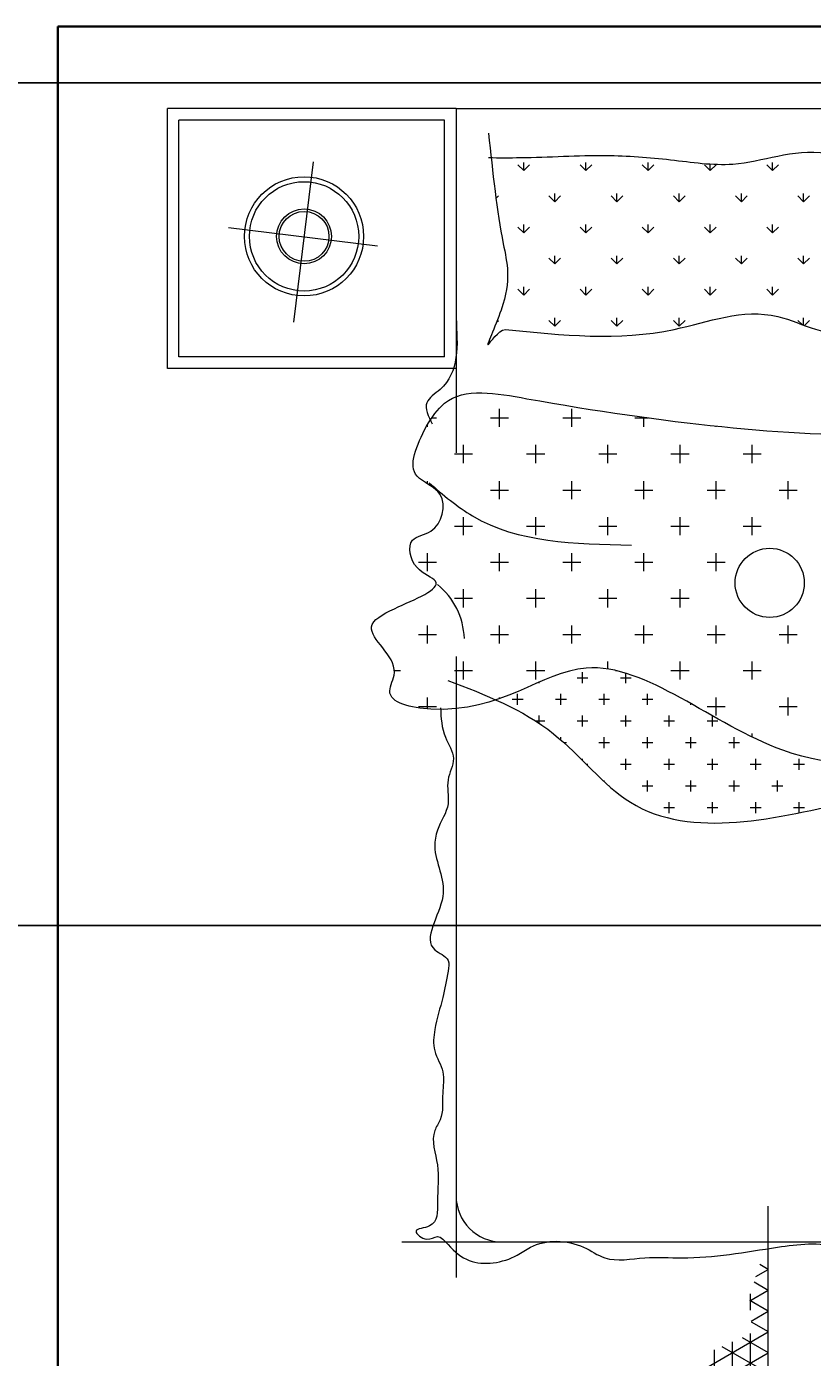
# Model space of a CAD drawing. Units: inches. Extents: x 3731 to 4318, y 1310 to 2388.
# Tile 26 of 57: x 3838 to 3894, y 1844 to 1938. Entities that reach past the tile are written whole.
import ezdxf

# ---------------------------------------------------------------- set-up
doc = ezdxf.new("R2010")
doc.units = ezdxf.units.IN
for name, color, linetype, lineweight in [('A-ANNO-DIMS', 2, 'Continuous', 18), ('A-FURN', 8, 'Continuous', 13), ('A-WALL', 7, 'Continuous', 35)]:
    doc.layers.add(name, color=color, linetype=linetype, lineweight=lineweight)
doc.styles.get("Standard").update_dxf_attribs({"font": 'arial.ttf'})
doc.dimstyles.get("Standard").update_dxf_attribs({"dimtxt": 0.18, "dimasz": 0.18, "dimexe": 0.18, "dimexo": 0.0625, "dimgap": 0.09, "dimtad": 0, "dimtih": 1, "dimtoh": 1, "dimdec": 4, "dimzin": 0, "dimdsep": 46, "dimtxsty": 'Standard', "dimcen": 0.09, "dimadec": 0, "dimazin": 0, "dimtfac": 1, "dimtdec": 4, "dimtofl": 0, "dimtmove": 0, "dimatfit": 3, "dimfxl": 1, "dimtolj": 1, "dimtzin": 0, "dimarcsym": 0})

# ---------------------------------------------------------------- blocks, each defined once
blk = doc.blocks.new('A$C200C7901')
for p, q in [((0, 1.8834), (0, 2.3334)), ((0.5, 2.3334), (0, 2.3334)), ((0.5, 2.3334), (0.5, 1.7369)), ((0.5, 2.3334), (0.5, 1.7369)), ((0.5, 2.3334), (2, 2.3334)), ((0.9943, 2.1721), (0.9842, 2.1822)), ((0.9943, 2.1721), (0.9842, 2.1822)), ((0.9943, 2.0643), (0.9842, 2.0744)), ((0.9943, 2.0643), (0.9842, 2.0744)), ((0.5701, 1.9635), (0.5733, 1.9666)), ((0.5701, 1.9635), (0.5733, 1.9666)), ((0.5, 1.8834), (0, 1.8834)), ((0.4504, 1.782), (0.4504, 1.7863)), ((0.4504, 1.782), (0.4504, 1.7863)), ((0.458, 1.7977), (0.466, 1.7977)), ((0.458, 1.7977), (0.466, 1.7977)), ((0.4504, 1.6834), (0.4504, 1.6883)), ((0.4504, 1.6834), (0.4504, 1.6883)), ((0.4656, 1.6727), (0.466, 1.6727)), ((0.4656, 1.6727), (0.466, 1.6727)), ((0.5597, 1.6727), (0.591, 1.6727)), ((0.5597, 1.6727), (0.591, 1.6727)), ((1.0129, 1.5945), (1.0129, 1.6258)), ((1.0129, 1.5945), (1.0129, 1.6258)), ((0.4347, 1.5477), (0.466, 1.5477)), ((0.4504, 1.532), (0.4504, 1.5633)), ((0.6847, 1.5477), (0.716, 1.5477)), ((1.0754, 1.5625), (1.0754, 1.5633)), ((1.0754, 1.5625), (1.0754, 1.5633)), ((0.4347, 1.4227), (0.466, 1.4227)), ((0.5, 1.3845), (0.5, 0.3086)), ((0.3931, 1.3602), (0.4035, 1.3602)), ((0.3931, 1.3602), (0.4035, 1.3602)), ((0.4972, 1.3602), (0.5285, 1.3602)), ((0.4972, 1.3602), (0.5285, 1.3602)), ((0.4347, 1.2977), (0.466, 1.2977)), ((0.4347, 1.2977), (0.466, 1.2977)), ((0.4504, 1.2936), (0.4504, 1.3133)), ((0.4504, 1.2936), (0.4504, 1.3133)), ((1.0407, 0.0275), (1.0407, 0.4323)), ((0.4061, 0.3703), (2.0386, 0.3703))]:
    blk.add_line(p, q)
at = {"linetype": 'ByBlock'}
for p, q in [((0.02, 1.9034), (0.02, 2.3134)), ((0.48, 2.3134), (0.02, 2.3134)), ((0.48, 1.9034), (0.48, 2.3134)), ((0.2524, 2.2412), (0.2186, 1.9635)), ((0.6171, 2.2259), (0.607, 2.236)), ((0.6171, 2.2259), (0.607, 2.236)), ((0.6171, 2.2259), (0.6171, 2.2402)), ((0.6171, 2.2259), (0.6171, 2.2402)), ((0.6171, 2.2259), (0.6272, 2.236)), ((0.6171, 2.2259), (0.6272, 2.236)), ((0.7249, 2.2259), (0.7148, 2.236)), ((0.7249, 2.2259), (0.7148, 2.236)), ((0.7249, 2.2259), (0.7249, 2.2402)), ((0.7249, 2.2259), (0.7249, 2.2402)), ((0.7249, 2.2259), (0.735, 2.236)), ((0.7249, 2.2259), (0.735, 2.236)), ((0.8326, 2.2259), (0.8225, 2.236)), ((0.8326, 2.2259), (0.8225, 2.236)), ((0.8326, 2.2259), (0.8326, 2.2402)), ((0.8326, 2.2259), (0.8326, 2.2402)), ((0.8326, 2.2259), (0.8427, 2.236)), ((0.8326, 2.2259), (0.8427, 2.236)), ((0.9404, 2.2259), (0.9303, 2.236)), ((0.9404, 2.2259), (0.9303, 2.236)), ((0.9404, 2.2259), (0.9404, 2.2369)), ((0.9404, 2.2259), (0.9404, 2.2369)), ((0.9404, 2.2259), (0.9505, 2.236)), ((0.9404, 2.2259), (0.9505, 2.236)), ((1.0482, 2.2259), (1.0381, 2.236)), ((1.0482, 2.2259), (1.0381, 2.236)), ((1.0482, 2.2259), (1.0482, 2.2402)), ((1.0482, 2.2259), (1.0482, 2.2402)), ((1.0482, 2.2259), (1.0583, 2.236)), ((1.0482, 2.2259), (1.0583, 2.236)), ((0.5692, 2.178), (0.5733, 2.1822)), ((0.5692, 2.178), (0.5733, 2.1822)), ((0.671, 2.1721), (0.6609, 2.1822)), ((0.671, 2.1721), (0.6609, 2.1822)), ((0.671, 2.172), (0.671, 2.1863)), ((0.671, 2.172), (0.671, 2.1863)), ((0.671, 2.1721), (0.6811, 2.1822)), ((0.671, 2.1721), (0.6811, 2.1822)), ((0.7787, 2.1721), (0.7686, 2.1822)), ((0.7787, 2.1721), (0.7686, 2.1822)), ((0.7787, 2.172), (0.7787, 2.1863)), ((0.7787, 2.172), (0.7787, 2.1863)), ((0.7787, 2.1721), (0.7889, 2.1822)), ((0.7787, 2.1721), (0.7889, 2.1822)), ((0.8865, 2.1721), (0.8764, 2.1822)), ((0.8865, 2.1721), (0.8764, 2.1822)), ((0.8865, 2.172), (0.8865, 2.1863)), ((0.8865, 2.172), (0.8865, 2.1863)), ((0.8865, 2.1721), (0.8966, 2.1822)), ((0.8865, 2.1721), (0.8966, 2.1822)), ((0.9943, 2.172), (0.9943, 2.1863)), ((0.9943, 2.172), (0.9943, 2.1863)), ((0.9943, 2.1721), (1.0044, 2.1822)), ((0.9943, 2.1721), (1.0044, 2.1822)), ((1.102, 2.1721), (1.0919, 2.1822)), ((1.102, 2.1721), (1.0919, 2.1822)), ((1.102, 2.172), (1.102, 2.1863)), ((1.102, 2.172), (1.102, 2.1863)), ((1.102, 2.1721), (1.1121, 2.1822)), ((1.102, 2.1721), (1.1121, 2.1822)), ((0.3641, 2.0951), (0.1061, 2.1268)), ((0.6171, 2.1182), (0.607, 2.1283)), ((0.6171, 2.1182), (0.607, 2.1283)), ((0.6171, 2.1182), (0.6171, 2.1325)), ((0.6171, 2.1182), (0.6171, 2.1325)), ((0.6171, 2.1182), (0.6272, 2.1283)), ((0.6171, 2.1182), (0.6272, 2.1283)), ((0.7249, 2.1182), (0.7148, 2.1283)), ((0.7249, 2.1182), (0.7148, 2.1283)), ((0.7249, 2.1182), (0.7249, 2.1325)), ((0.7249, 2.1182), (0.7249, 2.1325)), ((0.7249, 2.1182), (0.735, 2.1283)), ((0.7249, 2.1182), (0.735, 2.1283)), ((0.8326, 2.1182), (0.8225, 2.1283)), ((0.8326, 2.1182), (0.8225, 2.1283)), ((0.8326, 2.1182), (0.8326, 2.1325)), ((0.8326, 2.1182), (0.8326, 2.1325)), ((0.8326, 2.1182), (0.8427, 2.1283)), ((0.8326, 2.1182), (0.8427, 2.1283)), ((0.9404, 2.1182), (0.9303, 2.1283)), ((0.9404, 2.1182), (0.9303, 2.1283)), ((0.9404, 2.1182), (0.9404, 2.1325)), ((0.9404, 2.1182), (0.9404, 2.1325)), ((0.9404, 2.1182), (0.9505, 2.1283)), ((0.9404, 2.1182), (0.9505, 2.1283)), ((1.0482, 2.1182), (1.0381, 2.1283)), ((1.0482, 2.1182), (1.0381, 2.1283)), ((1.0482, 2.1182), (1.0482, 2.1325)), ((1.0482, 2.1182), (1.0482, 2.1325)), ((1.0482, 2.1182), (1.0583, 2.1283)), ((1.0482, 2.1182), (1.0583, 2.1283)), ((0.671, 2.0643), (0.671, 2.0786)), ((0.671, 2.0643), (0.671, 2.0786)), ((0.7787, 2.0643), (0.7787, 2.0786)), ((0.7787, 2.0643), (0.7787, 2.0786)), ((0.8865, 2.0643), (0.8865, 2.0786)), ((0.8865, 2.0643), (0.8865, 2.0786)), ((0.9943, 2.0643), (0.9943, 2.0786)), ((0.9943, 2.0643), (0.9943, 2.0786)), ((1.102, 2.0643), (1.102, 2.0786)), ((1.102, 2.0643), (1.102, 2.0786)), ((0.671, 2.0643), (0.6609, 2.0744)), ((0.671, 2.0643), (0.6609, 2.0744)), ((0.671, 2.0643), (0.6811, 2.0744)), ((0.671, 2.0643), (0.6811, 2.0744)), ((0.7787, 2.0643), (0.7686, 2.0744)), ((0.7787, 2.0643), (0.7686, 2.0744)), ((0.7787, 2.0643), (0.7889, 2.0744)), ((0.7787, 2.0643), (0.7889, 2.0744)), ((0.8865, 2.0643), (0.8764, 2.0744)), ((0.8865, 2.0643), (0.8764, 2.0744)), ((0.8865, 2.0643), (0.8966, 2.0744)), ((0.8865, 2.0643), (0.8966, 2.0744)), ((0.9943, 2.0643), (1.0044, 2.0744)), ((0.9943, 2.0643), (1.0044, 2.0744)), ((1.102, 2.0643), (1.0919, 2.0744)), ((1.102, 2.0643), (1.0919, 2.0744)), ((1.102, 2.0643), (1.1121, 2.0744)), ((1.102, 2.0643), (1.1121, 2.0744)), ((0.6171, 2.0104), (0.607, 2.0205)), ((0.6171, 2.0104), (0.607, 2.0205)), ((0.6171, 2.0104), (0.6171, 2.0247)), ((0.6171, 2.0104), (0.6171, 2.0247)), ((0.6171, 2.0104), (0.6272, 2.0205)), ((0.6171, 2.0104), (0.6272, 2.0205)), ((0.7249, 2.0104), (0.7148, 2.0205)), ((0.7249, 2.0104), (0.7148, 2.0205)), ((0.7249, 2.0104), (0.7249, 2.0247)), ((0.7249, 2.0104), (0.7249, 2.0247)), ((0.7249, 2.0104), (0.735, 2.0205)), ((0.7249, 2.0104), (0.735, 2.0205)), ((0.8326, 2.0104), (0.8225, 2.0205)), ((0.8326, 2.0104), (0.8225, 2.0205)), ((0.8326, 2.0104), (0.8326, 2.0247)), ((0.8326, 2.0104), (0.8326, 2.0247)), ((0.8326, 2.0104), (0.8427, 2.0205)), ((0.8326, 2.0104), (0.8427, 2.0205)), ((0.9404, 2.0104), (0.9303, 2.0205)), ((0.9404, 2.0104), (0.9303, 2.0205)), ((0.9404, 2.0104), (0.9404, 2.0247)), ((0.9404, 2.0104), (0.9404, 2.0247)), ((0.9404, 2.0104), (0.9505, 2.0205)), ((0.9404, 2.0104), (0.9505, 2.0205)), ((1.0482, 2.0104), (1.0381, 2.0205)), ((1.0482, 2.0104), (1.0381, 2.0205)), ((1.0482, 2.0104), (1.0482, 2.0247)), ((1.0482, 2.0104), (1.0482, 2.0247)), ((1.0482, 2.0104), (1.0583, 2.0205)), ((1.0482, 2.0104), (1.0583, 2.0205)), ((0.671, 1.9565), (0.6609, 1.9666)), ((0.671, 1.9565), (0.6609, 1.9666)), ((0.671, 1.9565), (0.671, 1.9708)), ((0.671, 1.9565), (0.671, 1.9708)), ((0.671, 1.9565), (0.6811, 1.9666)), ((0.671, 1.9565), (0.6811, 1.9666)), ((0.7787, 1.9565), (0.7686, 1.9666)), ((0.7787, 1.9565), (0.7686, 1.9666)), ((0.7787, 1.9565), (0.7787, 1.9708)), ((0.7787, 1.9565), (0.7787, 1.9708)), ((0.7787, 1.9565), (0.7889, 1.9666)), ((0.7787, 1.9565), (0.7889, 1.9666)), ((0.8865, 1.9565), (0.8764, 1.9666)), ((0.8865, 1.9565), (0.8764, 1.9666)), ((0.8865, 1.9565), (0.8865, 1.9708)), ((0.8865, 1.9565), (0.8865, 1.9708)), ((0.8865, 1.9565), (0.8966, 1.9666)), ((0.8865, 1.9565), (0.8966, 1.9666)), ((1.0993, 1.9593), (1.0919, 1.9666)), ((1.0993, 1.9593), (1.0919, 1.9666)), ((1.102, 1.9583), (1.102, 1.9708)), ((1.102, 1.9583), (1.102, 1.9708)), ((1.1033, 1.9578), (1.1121, 1.9666)), ((1.1033, 1.9578), (1.1121, 1.9666)), ((0.48, 1.9034), (0.02, 1.9034)), ((0.5754, 1.782), (0.5754, 1.8133)), ((0.5754, 1.782), (0.5754, 1.8133)), ((0.7004, 1.782), (0.7004, 1.8133)), ((0.7004, 1.782), (0.7004, 1.8133)), ((0.8254, 1.782), (0.8254, 1.7987)), ((0.8254, 1.782), (0.8254, 1.7987)), ((0.5597, 1.7977), (0.591, 1.7977)), ((0.5597, 1.7977), (0.591, 1.7977)), ((0.6847, 1.7977), (0.716, 1.7977)), ((0.6847, 1.7977), (0.716, 1.7977)), ((0.8097, 1.7977), (0.8331, 1.7977)), ((0.8097, 1.7977), (0.8331, 1.7977)), ((0.9504, 1.782), (0.9504, 1.7836)), ((0.9504, 1.782), (0.9504, 1.7836)), ((0.4972, 1.7352), (0.5285, 1.7352)), ((0.4972, 1.7352), (0.5285, 1.7352)), ((0.5129, 1.7195), (0.5129, 1.7508)), ((0.5129, 1.7195), (0.5129, 1.7508)), ((0.6222, 1.7352), (0.6535, 1.7352)), ((0.6222, 1.7352), (0.6535, 1.7352)), ((0.6379, 1.7195), (0.6379, 1.7508)), ((0.6379, 1.7195), (0.6379, 1.7508)), ((0.7472, 1.7352), (0.7785, 1.7352)), ((0.7472, 1.7352), (0.7785, 1.7352)), ((0.7629, 1.7195), (0.7629, 1.7508)), ((0.7629, 1.7195), (0.7629, 1.7508)), ((0.8722, 1.7352), (0.9035, 1.7352)), ((0.8722, 1.7352), (0.9035, 1.7352)), ((0.8879, 1.7195), (0.8879, 1.7508)), ((0.8879, 1.7195), (0.8879, 1.7508)), ((0.9972, 1.7352), (1.0285, 1.7352)), ((0.9972, 1.7352), (1.0285, 1.7352)), ((1.0129, 1.7195), (1.0129, 1.7508)), ((1.0129, 1.7195), (1.0129, 1.7508)), ((0.5754, 1.657), (0.5754, 1.6883)), ((0.5754, 1.657), (0.5754, 1.6883)), ((0.7004, 1.657), (0.7004, 1.6883)), ((0.7004, 1.657), (0.7004, 1.6883)), ((0.8254, 1.657), (0.8254, 1.6883)), ((0.8254, 1.657), (0.8254, 1.6883)), ((0.9504, 1.657), (0.9504, 1.6883)), ((0.9504, 1.657), (0.9504, 1.6883)), ((1.0754, 1.657), (1.0754, 1.6883)), ((1.0754, 1.657), (1.0754, 1.6883)), ((0.6847, 1.6727), (0.716, 1.6727)), ((0.6847, 1.6727), (0.716, 1.6727)), ((0.8097, 1.6727), (0.841, 1.6727)), ((0.8097, 1.6727), (0.841, 1.6727)), ((0.9347, 1.6727), (0.966, 1.6727)), ((0.9347, 1.6727), (0.966, 1.6727)), ((1.0597, 1.6727), (1.091, 1.6727)), ((1.0597, 1.6727), (1.091, 1.6727)), ((0.5129, 1.5945), (0.5129, 1.6258)), ((0.5129, 1.5945), (0.5129, 1.6258)), ((0.6379, 1.5945), (0.6379, 1.6258)), ((0.6379, 1.5945), (0.6379, 1.6258)), ((0.7629, 1.5945), (0.7629, 1.6258)), ((0.7629, 1.5945), (0.7629, 1.6258)), ((0.8879, 1.5945), (0.8879, 1.6258)), ((0.8879, 1.5945), (0.8879, 1.6258)), ((0.4972, 1.6102), (0.5285, 1.6102)), ((0.4972, 1.6102), (0.5285, 1.6102)), ((0.6222, 1.6102), (0.6535, 1.6102)), ((0.6222, 1.6102), (0.6535, 1.6102)), ((0.7472, 1.6102), (0.7785, 1.6102)), ((0.7472, 1.6102), (0.7785, 1.6102)), ((0.8722, 1.6102), (0.9035, 1.6102)), ((0.8722, 1.6102), (0.9035, 1.6102)), ((0.9972, 1.6102), (1.0285, 1.6102)), ((0.9972, 1.6102), (1.0285, 1.6102)), ((0.4347, 1.5477), (0.466, 1.5477)), ((0.4504, 1.532), (0.4504, 1.5633)), ((0.5597, 1.5477), (0.591, 1.5477)), ((0.5597, 1.5477), (0.591, 1.5477)), ((0.5754, 1.532), (0.5754, 1.5633)), ((0.5754, 1.532), (0.5754, 1.5633)), ((0.6847, 1.5477), (0.716, 1.5477)), ((0.7004, 1.532), (0.7004, 1.5633)), ((0.7004, 1.532), (0.7004, 1.5633)), ((0.8097, 1.5477), (0.841, 1.5477)), ((0.8097, 1.5477), (0.841, 1.5477)), ((0.8254, 1.532), (0.8254, 1.5633)), ((0.8254, 1.532), (0.8254, 1.5633)), ((0.9347, 1.5477), (0.966, 1.5477)), ((0.9347, 1.5477), (0.966, 1.5477)), ((0.9504, 1.532), (0.9504, 1.5633)), ((0.9504, 1.532), (0.9504, 1.5633)), ((0.5129, 1.4695), (0.5129, 1.5008)), ((0.5129, 1.4695), (0.5129, 1.5008)), ((0.6379, 1.4695), (0.6379, 1.5008)), ((0.6379, 1.4695), (0.6379, 1.5008)), ((0.7629, 1.4695), (0.7629, 1.5008)), ((0.7629, 1.4695), (0.7629, 1.5008)), ((0.8879, 1.4695), (0.8879, 1.5008)), ((0.8879, 1.4695), (0.8879, 1.5008)), ((0.4972, 1.4852), (0.5285, 1.4852)), ((0.4972, 1.4852), (0.5285, 1.4852)), ((0.6222, 1.4852), (0.6535, 1.4852)), ((0.6222, 1.4852), (0.6535, 1.4852)), ((0.7472, 1.4852), (0.7785, 1.4852)), ((0.7472, 1.4852), (0.7785, 1.4852)), ((0.8722, 1.4852), (0.9035, 1.4852)), ((0.8722, 1.4852), (0.9035, 1.4852)), ((0.4504, 1.407), (0.4504, 1.4383)), ((0.4504, 1.407), (0.4504, 1.4383)), ((0.5754, 1.407), (0.5754, 1.4383)), ((0.5754, 1.407), (0.5754, 1.4383)), ((0.7004, 1.407), (0.7004, 1.4383)), ((0.7004, 1.407), (0.7004, 1.4383)), ((0.8254, 1.407), (0.8254, 1.4383)), ((0.8254, 1.407), (0.8254, 1.4383)), ((0.9504, 1.407), (0.9504, 1.4383)), ((0.9504, 1.407), (0.9504, 1.4383)), ((1.0754, 1.407), (1.0754, 1.4383)), ((1.0754, 1.407), (1.0754, 1.4383)), ((0.4347, 1.4227), (0.466, 1.4227)), ((0.5597, 1.4227), (0.591, 1.4227)), ((0.5597, 1.4227), (0.591, 1.4227)), ((0.6847, 1.4227), (0.716, 1.4227)), ((0.6847, 1.4227), (0.716, 1.4227)), ((0.8097, 1.4227), (0.841, 1.4227)), ((0.8097, 1.4227), (0.841, 1.4227)), ((0.9347, 1.4227), (0.966, 1.4227)), ((0.9347, 1.4227), (0.966, 1.4227)), ((1.0597, 1.4227), (1.091, 1.4227)), ((1.0597, 1.4227), (1.091, 1.4227)), ((0.5129, 1.3445), (0.5129, 1.3758)), ((0.5129, 1.3445), (0.5129, 1.3758)), ((0.6222, 1.3602), (0.6535, 1.3602)), ((0.6222, 1.3602), (0.6535, 1.3602)), ((0.6379, 1.3445), (0.6379, 1.3758)), ((0.6379, 1.3445), (0.6379, 1.3758)), ((0.7629, 1.3627), (0.7629, 1.3758)), ((0.7629, 1.3627), (0.7629, 1.3758)), ((0.7762, 1.3602), (0.7785, 1.3602)), ((0.7762, 1.3602), (0.7785, 1.3602)), ((0.8722, 1.3602), (0.9035, 1.3602)), ((0.8722, 1.3602), (0.9035, 1.3602)), ((0.8879, 1.3445), (0.8879, 1.3758)), ((0.8879, 1.3445), (0.8879, 1.3758)), ((0.9972, 1.3602), (1.0285, 1.3602)), ((0.9972, 1.3602), (1.0285, 1.3602)), ((1.0129, 1.3445), (1.0129, 1.3758)), ((1.0129, 1.3445), (1.0129, 1.3758)), ((0.6441, 1.3383), (0.6441, 1.3399)), ((0.6441, 1.3383), (0.6441, 1.3399)), ((0.7097, 1.3477), (0.7285, 1.3477)), ((0.7097, 1.3477), (0.7285, 1.3477)), ((0.7191, 1.3383), (0.7191, 1.357)), ((0.7191, 1.3383), (0.7191, 1.357)), ((0.7847, 1.3477), (0.8035, 1.3477)), ((0.7847, 1.3477), (0.8035, 1.3477)), ((0.7941, 1.3383), (0.7941, 1.3554)), ((0.7941, 1.3383), (0.7941, 1.3554)), ((0.6066, 1.3008), (0.6066, 1.3195)), ((0.6066, 1.3008), (0.6066, 1.3195)), ((0.6816, 1.3008), (0.6816, 1.3195)), ((0.6816, 1.3008), (0.6816, 1.3195)), ((0.7566, 1.3008), (0.7566, 1.3195)), ((0.7566, 1.3008), (0.7566, 1.3195)), ((0.8316, 1.3008), (0.8316, 1.3195)), ((0.8316, 1.3008), (0.8316, 1.3195)), ((0.5754, 1.3115), (0.5754, 1.3133)), ((0.5754, 1.3115), (0.5754, 1.3133)), ((0.5972, 1.3102), (0.616, 1.3102)), ((0.5972, 1.3102), (0.616, 1.3102)), ((0.6722, 1.3102), (0.691, 1.3102)), ((0.6722, 1.3102), (0.691, 1.3102)), ((0.7472, 1.3102), (0.766, 1.3102)), ((0.7472, 1.3102), (0.766, 1.3102)), ((0.8222, 1.3102), (0.841, 1.3102)), ((0.8222, 1.3102), (0.841, 1.3102)), ((0.9066, 1.3008), (0.9066, 1.3028)), ((0.9066, 1.3008), (0.9066, 1.3028)), ((0.9347, 1.2977), (0.966, 1.2977)), ((0.9347, 1.2977), (0.966, 1.2977)), ((0.9504, 1.282), (0.9504, 1.3133)), ((0.9504, 1.282), (0.9504, 1.3133)), ((1.0597, 1.2977), (1.091, 1.2977)), ((1.0597, 1.2977), (1.091, 1.2977)), ((1.0754, 1.282), (1.0754, 1.3133)), ((1.0754, 1.282), (1.0754, 1.3133)), ((0.6379, 1.2727), (0.6535, 1.2727)), ((0.6379, 1.2727), (0.6535, 1.2727)), ((0.6441, 1.2686), (0.6441, 1.282)), ((0.6441, 1.2686), (0.6441, 1.282)), ((0.7097, 1.2727), (0.7285, 1.2727)), ((0.7097, 1.2727), (0.7285, 1.2727)), ((0.7191, 1.2633), (0.7191, 1.282)), ((0.7191, 1.2633), (0.7191, 1.282)), ((0.7847, 1.2727), (0.8035, 1.2727)), ((0.7847, 1.2727), (0.8035, 1.2727)), ((0.7941, 1.2633), (0.7941, 1.282)), ((0.7941, 1.2633), (0.7941, 1.282)), ((0.8597, 1.2727), (0.8785, 1.2727)), ((0.8597, 1.2727), (0.8785, 1.2727)), ((0.8691, 1.2633), (0.8691, 1.282)), ((0.8691, 1.2633), (0.8691, 1.282)), ((0.9347, 1.2727), (0.9535, 1.2727)), ((0.9347, 1.2727), (0.9535, 1.2727)), ((0.9441, 1.2633), (0.9441, 1.2816)), ((0.9441, 1.2633), (0.9441, 1.2816)), ((1.0129, 1.2448), (1.0129, 1.2508)), ((1.0129, 1.2448), (1.0129, 1.2508)), ((0.6816, 1.2398), (0.6816, 1.2445)), ((0.6816, 1.2398), (0.6816, 1.2445)), ((0.6868, 1.2352), (0.691, 1.2352)), ((0.6868, 1.2352), (0.691, 1.2352)), ((0.7472, 1.2352), (0.766, 1.2352)), ((0.7472, 1.2352), (0.766, 1.2352)), ((0.7566, 1.2258), (0.7566, 1.2445)), ((0.7566, 1.2258), (0.7566, 1.2445)), ((0.8222, 1.2352), (0.841, 1.2352)), ((0.8222, 1.2352), (0.841, 1.2352)), ((0.8316, 1.2258), (0.8316, 1.2445)), ((0.8316, 1.2258), (0.8316, 1.2445)), ((0.8972, 1.2352), (0.916, 1.2352)), ((0.8972, 1.2352), (0.916, 1.2352)), ((0.9066, 1.2258), (0.9066, 1.2445)), ((0.9066, 1.2258), (0.9066, 1.2445)), ((0.9722, 1.2352), (0.991, 1.2352)), ((0.9722, 1.2352), (0.991, 1.2352)), ((0.9816, 1.2258), (0.9816, 1.2445)), ((0.9816, 1.2258), (0.9816, 1.2445)), ((0.7191, 1.2041), (0.7191, 1.207)), ((0.7191, 1.2041), (0.7191, 1.207)), ((0.7941, 1.1883), (0.7941, 1.207)), ((0.7941, 1.1883), (0.7941, 1.207)), ((0.8691, 1.1883), (0.8691, 1.207)), ((0.8691, 1.1883), (0.8691, 1.207)), ((0.9441, 1.1883), (0.9441, 1.207)), ((0.9441, 1.1883), (0.9441, 1.207)), ((1.0191, 1.1883), (1.0191, 1.207)), ((1.0191, 1.1883), (1.0191, 1.207)), ((1.0941, 1.1883), (1.0941, 1.207)), ((1.0941, 1.1883), (1.0941, 1.207)), ((0.7255, 1.1977), (0.7285, 1.1977)), ((0.7255, 1.1977), (0.7285, 1.1977)), ((0.7847, 1.1977), (0.8035, 1.1977)), ((0.7847, 1.1977), (0.8035, 1.1977)), ((0.8597, 1.1977), (0.8785, 1.1977)), ((0.8597, 1.1977), (0.8785, 1.1977)), ((0.9347, 1.1977), (0.9535, 1.1977)), ((0.9347, 1.1977), (0.9535, 1.1977)), ((1.0097, 1.1977), (1.0285, 1.1977)), ((1.0097, 1.1977), (1.0285, 1.1977)), ((1.0847, 1.1977), (1.1035, 1.1977)), ((1.0847, 1.1977), (1.1035, 1.1977)), ((0.7566, 1.1674), (0.7566, 1.1695)), ((0.7566, 1.1674), (0.7566, 1.1695)), ((0.7646, 1.1602), (0.766, 1.1602)), ((0.7646, 1.1602), (0.766, 1.1602)), ((0.8222, 1.1602), (0.841, 1.1602)), ((0.8222, 1.1602), (0.841, 1.1602)), ((0.8316, 1.1508), (0.8316, 1.1695)), ((0.8316, 1.1508), (0.8316, 1.1695)), ((0.8972, 1.1602), (0.916, 1.1602)), ((0.8972, 1.1602), (0.916, 1.1602)), ((0.9066, 1.1508), (0.9066, 1.1695)), ((0.9066, 1.1508), (0.9066, 1.1695)), ((0.9722, 1.1602), (0.991, 1.1602)), ((0.9722, 1.1602), (0.991, 1.1602)), ((0.9816, 1.1508), (0.9816, 1.1695)), ((0.9816, 1.1508), (0.9816, 1.1695)), ((1.0472, 1.1602), (1.066, 1.1602)), ((1.0472, 1.1602), (1.066, 1.1602)), ((1.0566, 1.1508), (1.0566, 1.1695)), ((1.0566, 1.1508), (1.0566, 1.1695)), ((0.8691, 1.1133), (0.8691, 1.132)), ((0.8691, 1.1133), (0.8691, 1.132)), ((0.9441, 1.1133), (0.9441, 1.132)), ((0.9441, 1.1133), (0.9441, 1.132)), ((1.0191, 1.1133), (1.0191, 1.132)), ((1.0191, 1.1133), (1.0191, 1.132)), ((1.0941, 1.1136), (1.0941, 1.132)), ((1.0941, 1.1136), (1.0941, 1.132)), ((0.8597, 1.1227), (0.8785, 1.1227)), ((0.8597, 1.1227), (0.8785, 1.1227)), ((0.9347, 1.1227), (0.9535, 1.1227)), ((0.9347, 1.1227), (0.9535, 1.1227)), ((1.0097, 1.1227), (1.0285, 1.1227)), ((1.0097, 1.1227), (1.0285, 1.1227)), ((1.0847, 1.1227), (1.1035, 1.1227)), ((1.0847, 1.1227), (1.1035, 1.1227)), ((1.0261, 0.3316), (1.0407, 0.3232)), ((1.0261, 0.3316), (1.0407, 0.3232)), ((1.0164, 0.3011), (1.0407, 0.2871)), ((1.0164, 0.3011), (1.0407, 0.2871)), ((1.0194, 0.3103), (1.0407, 0.3227)), ((1.0194, 0.3103), (1.0407, 0.3227)), ((1.0089, 0.2682), (1.0407, 0.2866)), ((1.0089, 0.2682), (1.0407, 0.2866)), ((1.0099, 0.2521), (1.0099, 0.2804)), ((1.0099, 0.2521), (1.0099, 0.2804)), ((1.0088, 0.2694), (1.0407, 0.251)), ((1.0088, 0.2694), (1.0407, 0.251)), ((1.0111, 0.2334), (1.0407, 0.2505)), ((1.0111, 0.2334), (1.0407, 0.2505)), ((1.0112, 0.232), (1.0407, 0.215)), ((1.0112, 0.232), (1.0407, 0.215)), ((0.9344, 0.153), (1.0407, 0.2144)), ((0.9344, 0.153), (1.0407, 0.2144)), ((1.0099, 0.0251), (1.0099, 0.2117)), ((1.0099, 0.0251), (1.0099, 0.2117)), ((0.9602, 0.1893), (1.0407, 0.1428)), ((0.9602, 0.1893), (1.0407, 0.1428)), ((0.9787, 0.0381), (0.9787, 0.1976)), ((0.9787, 0.0381), (0.9787, 0.1976)), ((0.9953, 0.2051), (1.0407, 0.1789)), ((0.9953, 0.2051), (1.0407, 0.1789)), ((0.9355, 0.1176), (1.0407, 0.1783)), ((0.9355, 0.1176), (1.0407, 0.1783)), ((0.9474, 0.0512), (0.9474, 0.1835)), ((0.9474, 0.0512), (0.9474, 0.1835))]:
    blk.add_line(p, q, dxfattribs=at)
for radius in [0.1032, 0.0947, 0.0475, 0.0432]:
    blk.add_circle((0.2367, 2.1121), radius, dxfattribs=at)
blk.add_circle((1.0433, 1.5119), 0.0599)
blk.add_arc((0.3888, 1.4113), 0.1256, 1.9962, 51.1646, dxfattribs=at)
for centre, radius, start, end in [((0.3888, 1.4113), 0.1256, 1.9962, 51.1646), ((0.58, 0.4503), 0.08, 180, 270)]:
    blk.add_arc(centre, radius, start, end)
for points, knots in [([(0.5562, 2.2908), (0.5634, 2.223), (0.5751, 2.1147), (0.6005, 2.0213), (0.5392, 1.8966), (0.5726, 1.9486), (0.5854, 1.951)], [0, 0, 0, 0, 193.119101, 308.278592, 371.468985, 410.593498, 410.593498, 410.593498, 410.593498]), ([(0.5854, 1.951), (0.6835, 1.9407), (0.8425, 1.9242), (1.0374, 2.0054), (1.1564, 1.9255), (1.2274, 1.9841), (1.2052, 2.0751), (1.1815, 2.152), (1.2176, 2.2368), (1.0992, 2.2731), (1.0008, 2.2255), (0.8698, 2.246), (0.7481, 2.2548), (0.6426, 2.2473), (0.5746, 2.2478), (0.5562, 2.2479)], [0, 0, 0, 0, 292.165466, 473.33038, 601.631673, 630.723769, 727.138505, 836.819956, 887.958136, 954.42438, 1118.989809, 1227.016542, 1338.750986, 1487.447361, 1542.751028, 1542.751028, 1542.751028, 1542.751028]), ([(0.4485, 1.7835), (0.4321, 1.7496), (0.4062, 1.6964), (0.49, 1.6713), (0.4719, 1.5969), (0.4123, 1.592), (0.4233, 1.5337), (0.4954, 1.5086), (0.4012, 1.4738), (0.3253, 1.4306), (0.4113, 1.3764), (0.3688, 1.3065), (0.5579, 1.2663), (0.741, 1.4533), (1.1127, 1.1109), (1.4811, 1.2478), (1.7885, 1.3492), (2.0357, 1.1637), (2.0748, 1.2974), (2.0876, 1.349), (2.0192, 1.3805), (2.0564, 1.4298), (2.0588, 1.4846), (1.9759, 1.5349), (2.1004, 1.5845), (2.0397, 1.6519), (1.971, 1.7053), (2.1104, 1.8981), (1.5946, 1.7967), (1.2448, 1.7472), (0.8129, 1.7935), (0.4953, 1.8548), (0.4582, 1.7983), (0.4485, 1.7835)], [0, 0, 0, 0, 88.420092, 139.08588, 204.302936, 239.695496, 287.801042, 327.365471, 412.960499, 463.626286, 552.059846, 584.668336, 662.614915, 940.993281, 1309.926334, 1844.022653, 1996.276242, 2316.43048, 2341.441004, 2404.707416, 2449.463774, 2514.680778, 2538.40571, 2613.031547, 2697.13096, 2760.903931, 2822.692699, 2945.47, 3215.060018, 3725.584917, 4361.974444, 4504.671998, 4555.32777, 4555.32777, 4555.32777, 4555.32777]), ([(0.4856, 1.3429), (0.5504, 1.3182), (0.6715, 1.2721), (0.8374, 1.0498), (1.1164, 1.1183), (1.3878, 1.1816), (1.5888, 1.1102), (1.8403, 1.1127), (1.9415, 1.2178), (2.0032, 1.2819)], [0, 0, 0, 0, 205.411753, 383.654933, 772.067458, 921.644661, 1226.793228, 1388.983508, 1642.292305, 1642.292305, 1642.292305, 1642.292305])]:
    blk.add_open_spline(points, degree=3, knots=knots)
for points, knots in [([(0.5, 1.9703), (0.5029, 1.9235), (0.5066, 1.8648), (0.4398, 1.8252), (0.452, 1.8005), (0.4585, 1.7872)], [0, 0, 0, 0, 126.315232, 158.854004, 196.789047, 196.789047, 196.789047, 196.789047]), ([(0.5, 1.9703), (0.5029, 1.9235), (0.5066, 1.8648), (0.4398, 1.8252), (0.452, 1.8005), (0.4585, 1.7872)], [0, 0, 0, 0, 126.315232, 158.854004, 196.789047, 196.789047, 196.789047, 196.789047]), ([(0.4532, 1.6853), (0.4776, 1.6644), (0.574, 1.582), (0.7055, 1.5794), (0.8037, 1.5774)], [0, 0, 0, 0, 94.920667, 374.457292, 374.457292, 374.457292, 374.457292]), ([(0.4532, 1.6853), (0.4776, 1.6644), (0.574, 1.582), (0.7055, 1.5794), (0.8037, 1.5774)], [0, 0, 0, 0, 94.920667, 374.457292, 374.457292, 374.457292, 374.457292]), ([(0.473, 1.2954), (0.4739, 1.2781), (0.4755, 1.2477), (0.5032, 1.2084), (0.4801, 1.1701), (0.4928, 1.1255), (0.4674, 1.0912), (0.4579, 1.0351), (0.501, 0.9724), (0.4311, 0.8832), (0.4902, 0.8637), (0.4843, 0.8288), (0.4774, 0.7906), (0.4625, 0.7457), (0.459, 0.6999), (0.4816, 0.6664), (0.4748, 0.625), (0.4791, 0.5889), (0.4533, 0.5528), (0.4738, 0.5004), (0.4658, 0.4502), (0.4696, 0.3946), (0.4189, 0.3935), (0.4493, 0.3684), (0.4694, 0.3857), (0.4922, 0.3576), (0.5297, 0.3262), (0.5917, 0.3353), (0.6454, 0.3754), (0.7083, 0.3741), (0.7643, 0.3328), (0.826, 0.346), (0.925, 0.3388), (1.0353, 0.3593), (1.1561, 0.3744), (1.2477, 0.3154), (1.3302, 0.3474), (1.4086, 0.3512), (1.5217, 0.3878), (1.6362, 0.3176), (1.7682, 0.3285), (1.8402, 0.3019), (1.9071, 0.3529), (1.9647, 0.3412), (2.0795, 0.2948), (2.0472, 0.3498), (2.0343, 0.3772), (2.0435, 0.43), (2.0109, 0.5782), (2.0746, 0.4643), (2.0805, 0.584), (2.0084, 0.5979), (2.0343, 0.6846), (2.0344, 0.746), (2.0293, 0.8096), (2.0489, 0.8545), (2.0652, 0.9218), (1.9842, 0.9297), (2.0007, 1.0162), (2.0367, 1.0585), (2.0367, 1.1102), (2.0457, 1.1647), (2.0226, 1.2084), (2.0234, 1.2306), (2.0236, 1.2352)], [0, 0, 0, 0, 51.660678, 90.967412, 128.902454, 170.303599, 219.852997, 247.834962, 336.321557, 429.35469, 458.821847, 477.222321, 524.135809, 581.038434, 617.839381, 657.146115, 693.947125, 740.178081, 760.753248, 820.731705, 885.133458, 928.777044, 953.563729, 976.574207, 995.553042, 1018.563482, 1064.584401, 1147.951297, 1174.787598, 1266.851571, 1308.018447, 1377.066427, 1441.511314, 1608.245014, 1714.11869, 1792.771707, 1913.247991, 1954.931389, 2029.864445, 2259.189419, 2305.221512, 2429.507982, 2456.344283, 2543.92595, 2627.925037, 2662.96218, 2687.736879, 2719.937755, 2839.540991, 2875.47895, 2953.681041, 2993.270313, 3066.872333, 3154.395764, 3200.397042, 3248.426375, 3312.828127, 3347.881398, 3444.484026, 3481.577522, 3518.665244, 3592.267265, 3644.719162, 3658.519501, 3658.519501, 3658.519501, 3658.519501])]:
    blk.add_open_spline(points, degree=3, knots=knots, dxfattribs=at)
blk = doc.blocks.new('*D45')
at = {"layer": 'A-ANNO-DIMS', "color": 0, "lineweight": -2, "transparency": 16777216}
for p, q in [((3969.146, 1934.382), (3731.412, 1934.382)), ((3731.592, 1934.202), (3731.592, 1904.563)), ((3731.592, 1874.562), (3731.592, 1904.2)), ((3969.146, 1874.382), (3731.412, 1874.382))]:
    blk.add_line(p, q, dxfattribs=at)
at = {"layer": 'A-ANNO-DIMS', "color": 0, "transparency": 16777216}
for points in [[(3731.562, 1934.202), (3731.622, 1934.202), (3731.592, 1934.382)], [(3731.562, 1874.562), (3731.622, 1874.562), (3731.592, 1874.382)]]:
    blk.add_solid(points, dxfattribs=at)
at = {"layer": 'Defpoints', "color": 0, "transparency": 16777216}
for p in [(3731.592, 1934.382), (3969.209, 1934.382), (3969.209, 1874.382)]:
    blk.add_point(p, dxfattribs=at)
at = {"layer": 'A-ANNO-DIMS', "color": 0, "transparency": 16777216, "insert": (3731.592, 1904.382), "char_height": 0.18, "attachment_point": 5}
blk.add_mtext('\\A1;60', dxfattribs=at)

msp = doc.modelspace()

# ---------------------------------------------------------------- linework, layer by layer
at = {"layer": 'A-WALL'}
for q in [(3960.209, 1938.382), (3840.209, 1779.382)]:
    msp.add_line((3840.209, 1938.382), q, dxfattribs=at)

# ---------------------------------------------------------------- block references
at = {"layer": 'A-FURN', "xscale": 41.1071563136412, "yscale": 41.1071563136412, "zscale": 41.1071563136412}
msp.add_blockref('A$C200C7901', (3848.004, 1836.625), dxfattribs=at)

# ---------------------------------------------------------------- dimensions: what is measured, and where the dimension line sits
at = {"layer": 'A-ANNO-DIMS'}
dim = msp.add_linear_dim(base=(3731.592, 1934.382), p1=(3969.209, 1874.382), p2=(3969.209, 1934.382), angle=90, dimstyle='Standard', override={"dimdec": 0, "dimlfac": 1, "dimrnd": 0, "dimzin": 0, "dimdsep": 46, "dimlunit": 2}, dxfattribs=at)
dim.commit()
dim.dimension.update_dxf_attribs({"geometry": '*D45', "text_midpoint": (3731.592, 1904.382)})

doc.saveas('drawing.dxf')
